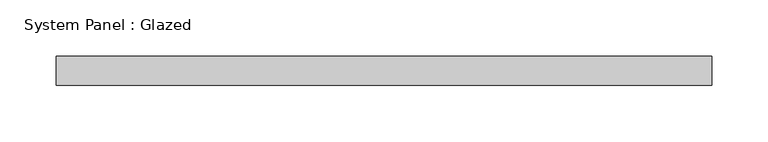
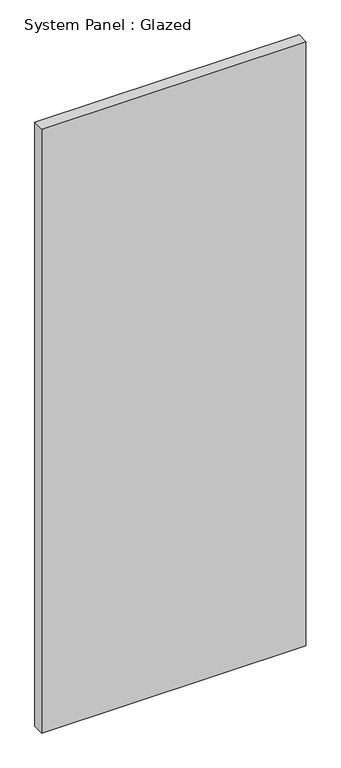
"""IFC4 building model written with IfcOpenShell, lengths in millimetres: plate geometry, System Panel : Glazed."""

from ifc_helpers import new_model, si_unit, origin, origin_with_axes, place, context, project, spatial, polyline, outline, extrude, source, transform, mapped, element, save


def system_panel_glazed_7c7839b8(model_context):
    return source(origin(), model_context, "Body", "SweptSolid", [
        extrude(outline(polyline([(290.5125, 19.05), (-290.5125, 19.05), (-290.5125, 44.45), (290.5125, 44.45), (290.5125, 19.05)])), origin_with_axes(), (0.0, 0.0, 1.0), 1404.3368617),
    ])


if __name__ == "__main__":
    model = new_model("IFC4")
    model_context = context("Model", 3, world=origin())
    ifc_project = project(units=[si_unit("LENGTHUNIT", "METRE", prefix="MILLI")], contexts=[model_context])
    site = spatial("IfcSite", under=ifc_project)
    building = spatial("IfcBuilding", under=site)
    placement = place(None, origin())
    system_panel_glazed_shape = system_panel_glazed_7c7839b8(model_context)
    element("IfcPlate", 1, ObjectType="System Panel : Glazed", at=placement, inside=building, context=model_context, shape_type="MappedRepresentation", body=[
        mapped(system_panel_glazed_shape, transform((0.0, 0.0, 0.0), x_axis=(1.0, 0.0, 0.0), y_axis=(0.0, 1.0, 0.0), z_axis=(0.0, 0.0, 1.0))),
    ])
    save(model, "model.ifc")

# Revit data of these elements
# Type "System Panel : Glazed"
#   Construction Type Id = "GSP4R"
#   Analytic Construction = "1/8 in Pilkington single glazing"
#   Visual Light Transmittance = 0.9
#   Solar Heat Gain Coefficient = 0.86
#   Heat Transfer Coefficient (U) = 1.18115 BTU/(h·ft²·°F)
#   Define Thermal Properties by = 1
# Element 1 (IfcPlate, "System Panel : Glazed")
#   Materials on its faces: "Glass"
# Materials
#   "Glass": class "Glass", colour RGB 0 128 192, transparency 0.75, Description = "Soda Lime Glass", Cost = 0
